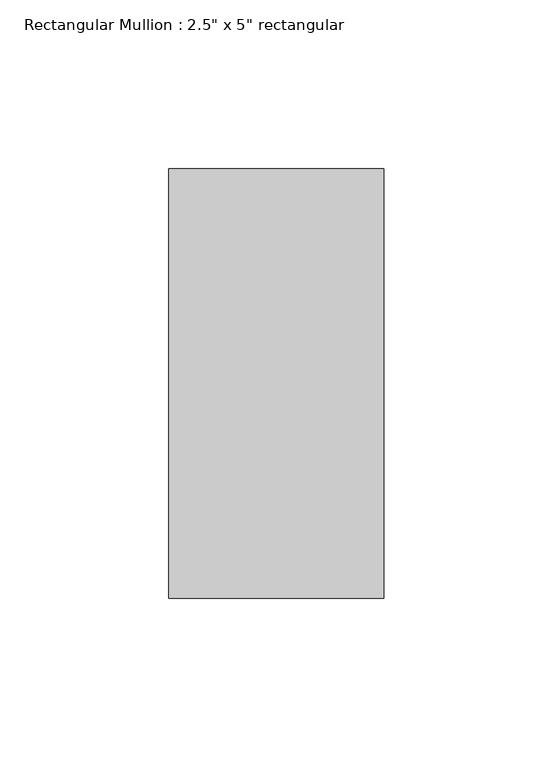
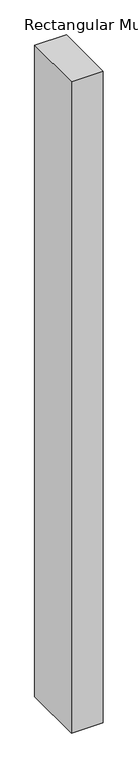
"""IFC4 building model written with IfcOpenShell, lengths in millimetres: member geometry."""

from ifc_helpers import new_model, si_unit, frame, origin, place, context, project, spatial, polyline, outline, extrude, source, transform, mapped, element, save


def member_55cf8d67(model_context):
    return source(origin(), model_context, "Body", "SweptSolid", [
        extrude(outline(polyline([(0.0, 63.5), (0.0, -63.5), (-63.5, -63.5), (-63.5, 63.5), (0.0, 63.5)])), frame((0.0, 0.0, -1378.4977008), z_axis=(0.0, 0.0, 1.0), x_axis=(1.0, 0.0, 0.0)), (0.0, 0.0, 1.0), 1378.4977008),
    ])


if __name__ == "__main__":
    model = new_model("IFC4")
    model_context = context("Model", 3, world=origin())
    ifc_project = project(units=[si_unit("LENGTHUNIT", "METRE", prefix="MILLI")], contexts=[model_context])
    site = spatial("IfcSite", under=ifc_project)
    building = spatial("IfcBuilding", under=site)
    placement = place(None, origin())
    member_shape = member_55cf8d67(model_context)
    element("IfcMember", 1, ObjectType="Rectangular Mullion : 2.5\" x 5\" rectangular", at=placement, inside=building, context=model_context, shape_type="MappedRepresentation", body=[
        mapped(member_shape, transform((0.0, 0.0, 0.0), x_axis=(1.0, 0.0, 0.0), y_axis=(0.0, 1.0, 0.0), z_axis=(0.0, 0.0, 1.0))),
    ])
    save(model, "model.ifc")

# Revit data of these elements
# Type "Rectangular Mullion : 2.5\" x 5\" rectangular"
#   built-in parameter 1007304 = 0.416667 (stored number, unit not read)
#   built-in parameter 1007301 = 0.104167 (stored number, unit not read)
#   built-in parameter 1007300 = 0.104167 (stored number, unit not read)
# Element 1 (IfcMember, "Rectangular Mullion : 2.5\" x 5\" rectangular")
#   Materials on its faces: "Aluminum"
# Materials
#   "Aluminum": class "Metal", colour RGB 247 247 247, transparency 0, Description = "Aluminum 6061", Cost = 0
